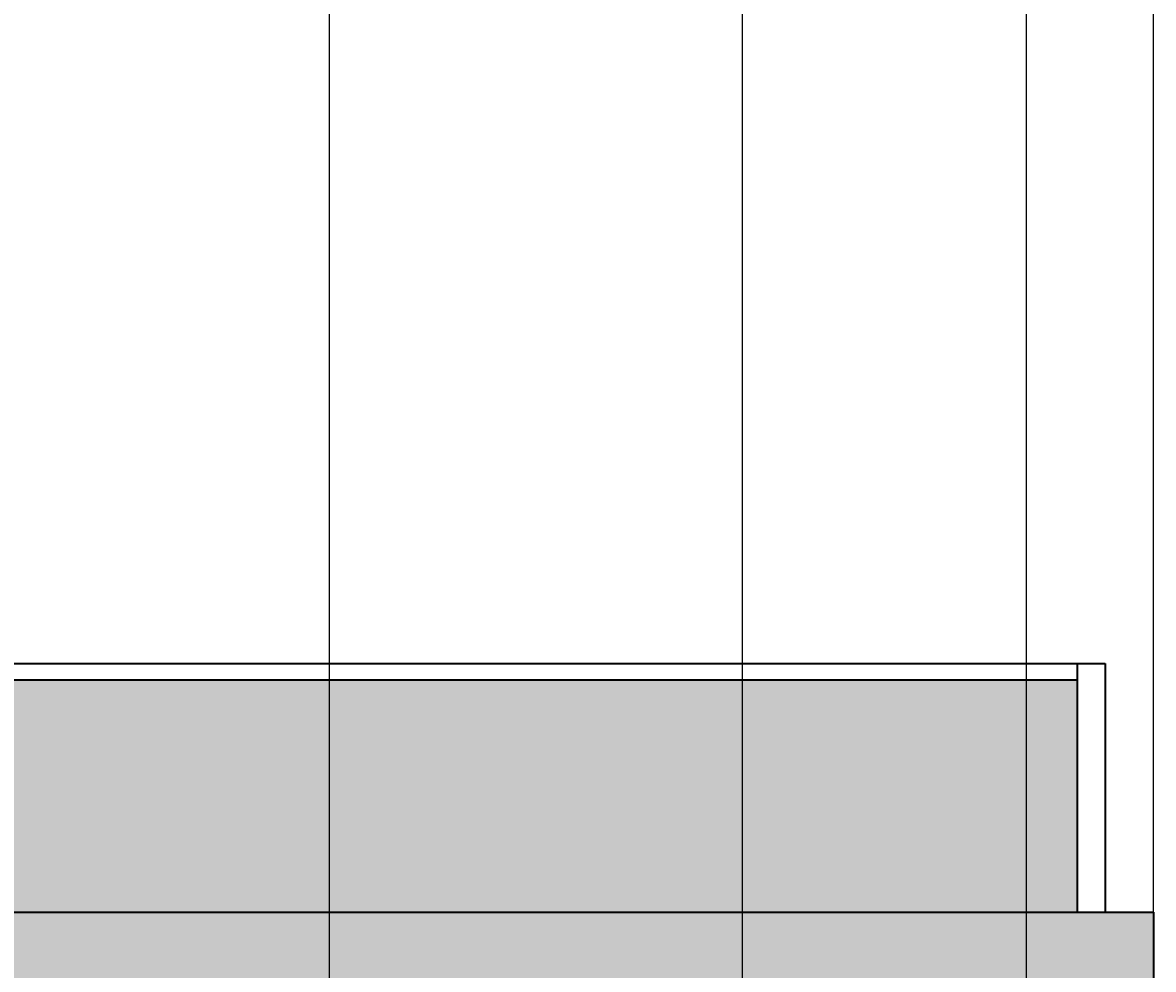
# Model space of a CAD drawing. Units: inches. Extents: x -5 to 714, y 84 to 644.
# Tile 18 of 20: x 457 to 593, y 308 to 423. Entities that reach past the tile are written whole.
import ezdxf

# ---------------------------------------------------------------- set-up
doc = ezdxf.new("R2010")
doc.units = ezdxf.units.IN
doc.header["$MEASUREMENT"] = 0
for name, color, linetype, lineweight in [('A-ANNO-DIMS', 2, 'Continuous', 18), ('A-ELEV', 7, 'Continuous', 35), ('A-ELEV-PATT', 8, 'Continuous', 13)]:
    doc.layers.add(name, color=color, linetype=linetype, lineweight=lineweight)
doc.styles.get("Standard").update_dxf_attribs({"font": 'arial.ttf'})
doc.dimstyles.get("Standard").update_dxf_attribs({"dimtxt": 0.9375, "dimasz": 0.18, "dimexe": 0.18, "dimexo": 0.0625, "dimgap": 0.09, "dimtad": 0, "dimtih": 1, "dimtoh": 1, "dimdec": 4, "dimzin": 0, "dimdsep": 46, "dimlunit": 4, "dimtxsty": 'Standard', "dimcen": 0.09, "dimadec": 0, "dimazin": 0, "dimtfac": 1, "dimtdec": 4, "dimtofl": 0, "dimtmove": 0, "dimatfit": 3, "dimfxl": 1, "dimtolj": 1, "dimtzin": 0, "dimarcsym": 0})

# ---------------------------------------------------------------- blocks, each defined once
blk = doc.blocks.new('*D54')
at = {"layer": 'A-ANNO-DIMS', "color": 0, "lineweight": -2, "transparency": 16777216}
for p, q in [((259.07, 315.16), (259.07, 643.61)), ((259.25, 643.43), (424.21, 643.43)), ((593.25, 643.43), (428.28, 643.43)), ((593.43, 315.16), (593.43, 643.61))]:
    blk.add_line(p, q, dxfattribs=at)
at = {"layer": 'A-ANNO-DIMS', "color": 0, "transparency": 16777216}
for points in [[(259.25, 643.46), (259.25, 643.4), (259.07, 643.43)], [(593.25, 643.46), (593.25, 643.4), (593.43, 643.43)]]:
    blk.add_solid(points, dxfattribs=at)
at = {"layer": 'Defpoints', "color": 0, "transparency": 16777216}
for p in [(593.43, 643.43), (259.07, 315.1), (593.43, 315.1)]:
    blk.add_point(p, dxfattribs=at)
at = {"layer": 'A-ANNO-DIMS', "color": 0, "transparency": 16777216, "insert": (426.25, 643.43), "char_height": 0.938, "attachment_point": 5}
blk.add_mtext('\\A1;334.36', dxfattribs=at)
blk = doc.blocks.new('*D62')
at = {"layer": 'A-ANNO-DIMS', "color": 0, "lineweight": -2, "transparency": 16777216}
for p, q in [((407.38, 266.06), (407.38, 643.61)), ((407.56, 643.43), (449.27, 643.43)), ((493.6, 643.43), (451.89, 643.43)), ((493.78, 266.06), (493.78, 643.61))]:
    blk.add_line(p, q, dxfattribs=at)
at = {"layer": 'A-ANNO-DIMS', "color": 0, "transparency": 16777216}
for points in [[(407.56, 643.46), (407.56, 643.4), (407.38, 643.43)], [(493.6, 643.46), (493.6, 643.4), (493.78, 643.43)]]:
    blk.add_solid(points, dxfattribs=at)
at = {"layer": 'Defpoints', "color": 0, "transparency": 16777216}
for p in [(493.78, 643.43), (407.38, 266), (493.78, 266)]:
    blk.add_point(p, dxfattribs=at)
at = {"layer": 'A-ANNO-DIMS', "color": 0, "transparency": 16777216, "insert": (450.58, 643.43), "char_height": 0.938, "attachment_point": 5}
blk.add_mtext('\\A1;86.4', dxfattribs=at)
blk = doc.blocks.new('*D63')
at = {"layer": 'A-ANNO-DIMS', "color": 0, "lineweight": -2, "transparency": 16777216}
for p, q in [((493.78, 266.06), (493.78, 643.61)), ((493.96, 643.43), (517.06, 643.43)), ((543.54, 643.43), (520.44, 643.43)), ((543.72, 266.06), (543.72, 643.61))]:
    blk.add_line(p, q, dxfattribs=at)
at = {"layer": 'A-ANNO-DIMS', "color": 0, "transparency": 16777216}
for points in [[(493.96, 643.46), (493.96, 643.4), (493.78, 643.43)], [(543.54, 643.46), (543.54, 643.4), (543.72, 643.43)]]:
    blk.add_solid(points, dxfattribs=at)
at = {"layer": 'Defpoints', "color": 0, "transparency": 16777216}
for p in [(543.72, 643.43), (493.78, 266), (543.72, 266)]:
    blk.add_point(p, dxfattribs=at)
at = {"layer": 'A-ANNO-DIMS', "color": 0, "transparency": 16777216, "insert": (518.75, 643.43), "char_height": 0.938, "attachment_point": 5}
blk.add_mtext('\\A1;49.94', dxfattribs=at)
blk = doc.blocks.new('*D64')
at = {"layer": 'A-ANNO-DIMS', "color": 0, "lineweight": -2, "transparency": 16777216}
for p, q in [((543.72, 266.06), (543.72, 643.61)), ((543.9, 643.43), (558.86, 643.43)), ((577.91, 643.43), (562.94, 643.43)), ((578.09, 277.11), (578.09, 643.61))]:
    blk.add_line(p, q, dxfattribs=at)
at = {"layer": 'A-ANNO-DIMS', "color": 0, "transparency": 16777216}
for points in [[(543.9, 643.46), (543.9, 643.4), (543.72, 643.43)], [(577.91, 643.46), (577.91, 643.4), (578.09, 643.43)]]:
    blk.add_solid(points, dxfattribs=at)
at = {"layer": 'Defpoints', "color": 0, "transparency": 16777216}
for p in [(578.09, 643.43), (578.09, 277.05), (543.72, 266)]:
    blk.add_point(p, dxfattribs=at)
at = {"layer": 'A-ANNO-DIMS', "color": 0, "transparency": 16777216, "insert": (560.9, 643.43), "char_height": 0.938, "attachment_point": 5}
blk.add_mtext('\\A1;34.375', dxfattribs=at)

msp = doc.modelspace()

# ---------------------------------------------------------------- hatches: boundary and pattern name
at = {"layer": 'A-ELEV-PATT', "transparency": 33554687}
h = msp.add_hatch(color=256, dxfattribs=at)
h.dxf.hatch_style = 1
h.paths.add_polyline_path([(188.3677, 525.1928), (67.9893, 525.1928), (67.9893, 489.1928), (67.9893, 345.1928), (126.7303, 345.1928), (126.7303, 480.1709), (229.3575, 480.1709), (229.3575, 525.1928), (212.6043, 525.1928), (212.6043, 482.7164), (211.0019, 482.7164), (211.0019, 525.1928), (207.6919, 525.1928), (199.9852, 525.1928), (199.9852, 482.7164), (198.3828, 482.7164), (198.3828, 525.1928), (189.9701, 525.1928), (189.9701, 482.7164), (188.3677, 482.7164)])
h.paths.add_polyline_path([(121.3589, 336.2066), (75.5048, 336.2066), (75.5048, 319.345), (121.3589, 319.345)])
h.paths.add_polyline_path([(121.3589, 319.345), (75.5048, 319.345), (75.5048, 302.3045), (121.3589, 302.3045)])
h.paths.add_polyline_path([(121.3589, 302.3045), (75.5048, 302.3045), (75.5048, 282.8561), (121.3589, 282.8561)])
h.paths.add_polyline_path([(121.3589, 282.8561), (75.5048, 282.8561), (75.5048, 261.5556), (121.3589, 261.5556)])
h.paths.add_polyline_path([(121.3589, 261.5556), (75.5048, 261.5556), (75.5048, 243.7009), (121.3589, 243.7009)])
h.paths.add_polyline_path([(121.3589, 243.7009), (75.5048, 243.7009), (75.5048, 223.5117), (121.3589, 223.5117)])
h.paths.add_polyline_path([(121.3589, 223.5117), (75.5048, 223.5117), (75.5048, 212.5836), (121.3589, 212.5836)])
h.paths.add_polyline_path([(121.3589, 212.5836), (75.5048, 212.5836), (75.5048, 201.1928), (121.3589, 201.1928)])
h.paths.add_polyline_path([(179.9335, 201.1928), (30.1395, 201.1928), (30.1395, 198.7054), (179.9335, 198.7054)])
h.paths.add_polyline_path([(187.6349, 201.1928), (179.9335, 201.1928), (179.9335, 198.7054), (179.9335, 141.1928), (269.2446, 141.1928), (269.2446, 201.1928), (263.4349, 201.1928), (263.4349, 152.1176), (187.6349, 152.1176)])
h.paths.add_polyline_path([(269.2446, 277.0513), (269.2446, 287.501), (269.2446, 306.6286), (578.0915, 306.6286), (578.0915, 201.1928), (593.428, 201.1928), (593.428, 315.0968), (584.4202, 315.0968), (259.0665, 315.0968), (259.0665, 201.1928), (263.4349, 201.1928), (269.2446, 201.1928)])
h = msp.add_hatch(color=256, dxfattribs=at)
h.dxf.hatch_style = 1
h.paths.add_polyline_path([(584.2229, 343.1928), (259.0665, 343.1928), (259.0665, 315.0968), (584.2229, 315.0968)])
h.paths.add_polyline_path([(352.9482, 258.2864), (332.0052, 258.2864), (332.0052, 201.1928), (352.9482, 201.1928)])
h.paths.add_polyline_path([(378.5957, 258.2864), (357.6527, 258.2864), (357.6527, 201.1928), (378.5957, 201.1928)])
h.paths.add_polyline_path([(403.4391, 258.2864), (382.4961, 258.2864), (382.4961, 201.1928), (403.4391, 201.1928)])
h.paths.add_polyline_path([(339.2672, 197.3754), (332.0052, 197.3754), (332.0052, 191.3028), (339.2672, 191.3028)])
h.paths.add_polyline_path([(352.9482, 197.3754), (343.9704, 197.3754), (343.9704, 191.3028), (352.9482, 191.3028)])
h.paths.add_polyline_path([(352.9482, 189.3028), (343.9704, 189.3028), (343.9704, 184.8307), (352.9482, 184.8307)])
h.paths.add_polyline_path([(339.2672, 189.3028), (332.0052, 189.3028), (332.0052, 184.8307), (339.2672, 184.8307)])
h.paths.add_polyline_path([(339.2672, 182.8307), (332.0052, 182.8307), (332.0052, 177.6504), (339.2672, 177.6504)])
h.paths.add_polyline_path([(352.9482, 182.8307), (343.9704, 182.8307), (343.9704, 177.6504), (352.9482, 177.6504)])
h.paths.add_polyline_path([(352.9482, 175.6504), (343.9704, 175.6504), (343.9704, 173.6169), (352.9482, 173.6169)])
h.paths.add_polyline_path([(339.2672, 175.6504), (332.0052, 175.6504), (332.0052, 173.6169), (339.2672, 173.6169)])
h.paths.add_polyline_path([(376.2796, 175.6504), (357.6527, 175.6504), (357.6527, 173.6169), (376.2796, 173.6169)])
h.paths.add_polyline_path([(376.2796, 182.8307), (357.6527, 182.8307), (357.6527, 177.6504), (376.2796, 177.6504)])
h.paths.add_polyline_path([(376.2796, 189.3028), (357.6527, 189.3028), (357.6527, 184.8307), (376.2796, 184.8307)])
h.paths.add_polyline_path([(376.2796, 197.3754), (357.6527, 197.3754), (357.6527, 191.3028), (376.2796, 191.3028)])
h.paths.add_polyline_path([(403.4391, 197.3754), (382.4961, 197.3754), (382.4961, 191.3028), (403.4391, 191.3028)])
h.paths.add_polyline_path([(403.4391, 189.3028), (382.4961, 189.3028), (382.4961, 184.8307), (403.4391, 184.8307)])
h.paths.add_polyline_path([(403.4391, 182.8307), (382.4961, 182.8307), (382.4961, 177.6504), (403.4391, 177.6504)])
h.paths.add_polyline_path([(403.4391, 175.6504), (382.4961, 175.6504), (382.4961, 173.6169), (403.4391, 173.6169)])

# ---------------------------------------------------------------- linework, layer by layer
at = {"layer": 'A-ELEV'}
for p, q in [((67.9893, 345.1928), (587.5794, 345.1928)), ((584.2229, 345.1928), (584.2229, 315.0968)), ((587.5794, 345.1928), (587.5794, 315.0968)), ((259.0665, 343.1928), (584.2229, 343.1928)), ((259.0665, 315.0968), (584.4202, 315.0968)), ((584.4202, 315.0968), (593.428, 315.0968)), ((593.428, 315.0968), (593.428, 201.1928))]:
    msp.add_line(p, q, dxfattribs=at)

# ---------------------------------------------------------------- dimensions: what is measured, and where the dimension line sits
at = {"layer": 'A-ANNO-DIMS'}
for base, p1, p2, override, picture, middle in [((593.428, 643.4276), (259.0665, 315.0968), (593.428, 315.0968), {"dimdec": 2, "dimlfac": 1, "dimrnd": 0, "dimzin": 0, "dimdsep": 46, "dimlunit": 2}, '*D54', (426.2472, 643.4276)), ((493.7771, 643.4276), (407.3813, 266.0021), (493.7771, 266.0021), {"dimdec": 1, "dimlfac": 1, "dimrnd": 0, "dimzin": 0, "dimdsep": 46, "dimlunit": 2}, '*D62', (450.5792, 643.4276)), ((543.7164, 643.4276), (493.7771, 266.0021), (543.7164, 266.0021), {"dimdec": 2, "dimlfac": 1, "dimrnd": 0, "dimzin": 0, "dimdsep": 46, "dimlunit": 2}, '*D63', (518.7468, 643.4276)), ((578.0915, 643.4276), (543.7164, 266.0021), (578.0915, 277.0513), {"dimdec": 3, "dimlfac": 1, "dimrnd": 0, "dimzin": 0, "dimdsep": 46, "dimlunit": 2}, '*D64', (560.904, 643.4276))]:
    dim = msp.add_linear_dim(base=base, p1=p1, p2=p2, dimstyle='Standard', override=override, dxfattribs=at)
    dim.commit()
    dim.dimension.update_dxf_attribs({"geometry": picture, "text_midpoint": middle})

doc.saveas('drawing.dxf')
